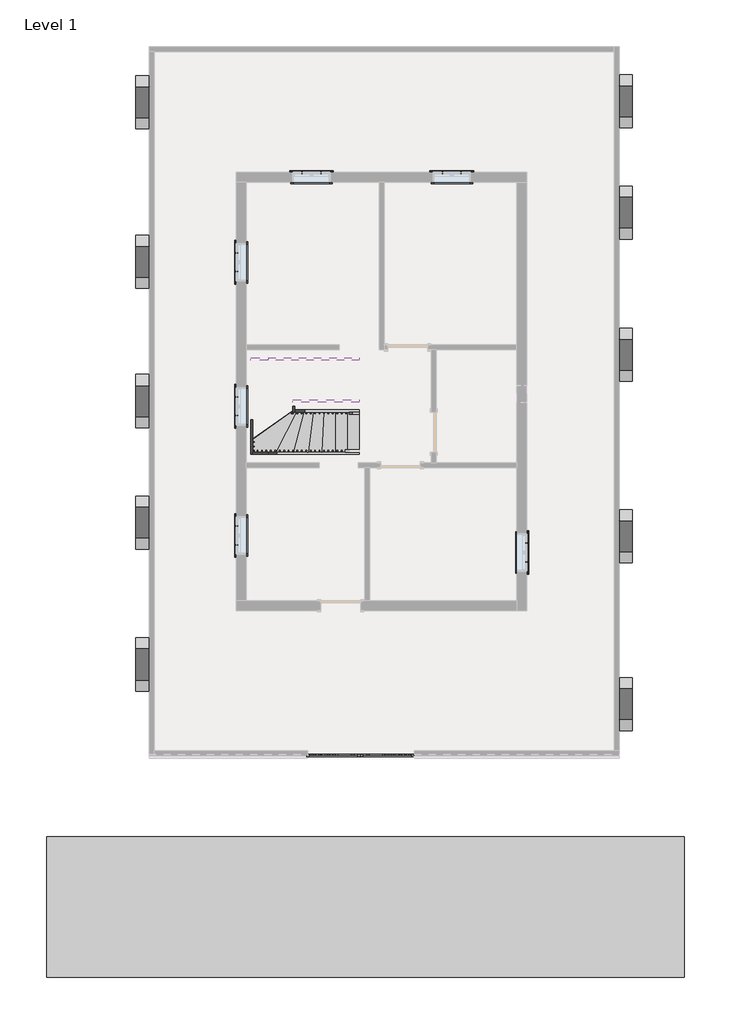
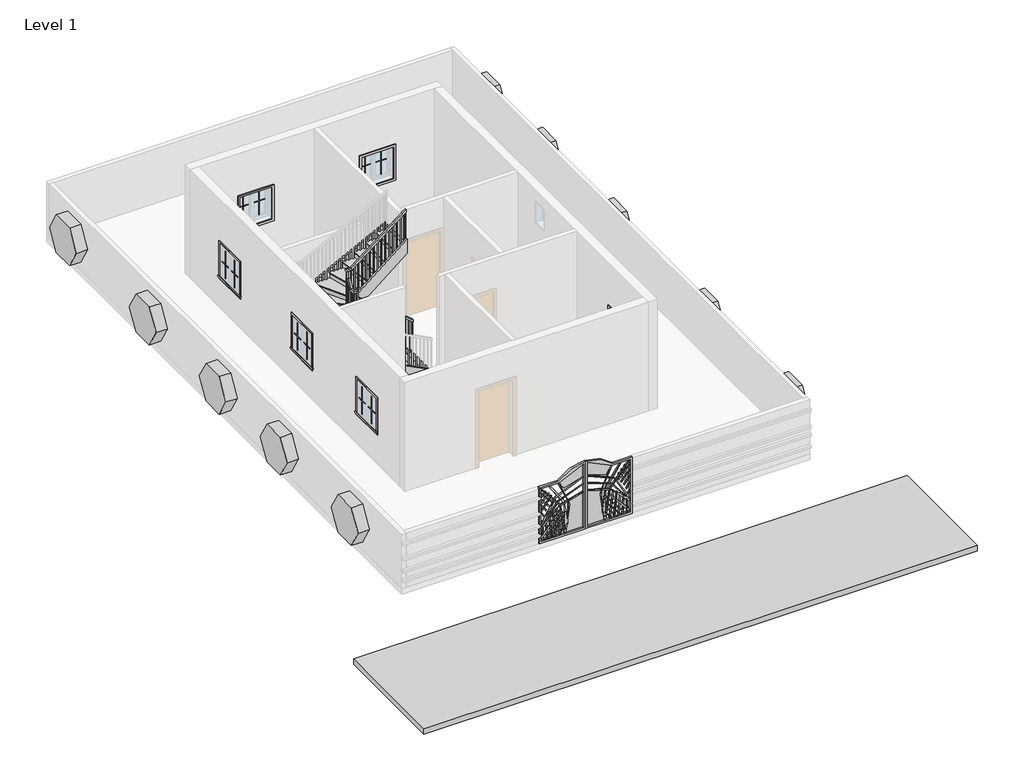
# One storey, part 3 of 3: 28 proxies, 8 members, 1 railing, 1 stair flight.
"""IFC4 building model written with IfcOpenShell, lengths in millimetres."""

from ifc_helpers import new_model, si_unit, frame, origin, place, context, project, spatial, polyline, outline, extrude, faceted_brep, transform, mapped, element, save
from components import generic_models_6bc30956, generic_models_2_generic_models_2_a0eb84b6, generic_models_3_generic_models_3_c1cfd057, generic_models_4_generic_models_4_ada6ec20, muntin_pattern_2x2_muntin_pattern_2x2_b3fe6957, muntin_pattern_2x2_muntin_pattern_2x2_3e0ecaf2, trim_window_exterior_flat_with_sill_41619996, trim_window_interior_flat_picture_frame_51c85655, stair_flight_6f16d7d9

model = new_model("IFC4")

# Units and contexts
model_context = context("Model", 3, world=origin())
ifc_project = project(units=[si_unit("LENGTHUNIT", "METRE", prefix="MILLI")], contexts=[model_context])

# Site, building, storey
site = spatial("IfcSite", under=ifc_project)
building = spatial("IfcBuilding", under=site)
storey = spatial("IfcBuildingStorey", under=building, Name="Level 1", Elevation=0.0)

# Proxies
placement = place(None, origin())
generic_models_shape = generic_models_6bc30956(model_context)
element("IfcBuildingElementProxy", 1, Name="Generic Models", at=placement, inside=storey, context=model_context, shape_type="MappedRepresentation", body=[
    mapped(generic_models_shape, transform((-1768.0949167, -8199.8056704, 0.0), x_axis=(1.0, 0.0, 0.0), y_axis=(0.0, 1.0, 0.0), z_axis=(0.0, 0.0, 1.0))),
])
generic_models_2_generic_models_2_shape = generic_models_2_generic_models_2_a0eb84b6(model_context)
element("IfcBuildingElementProxy", 2, Name="Generic Models 2 : Generic Models 2", ObjectType="Generic Models 2 : Generic Models 2", at=placement, inside=storey, context=model_context, shape_type="MappedRepresentation", body=[
    mapped(generic_models_2_generic_models_2_shape, transform((0.0, 0.0, 0.0), x_axis=(1.0, 0.0, 0.0), y_axis=(0.0, 1.0, 0.0), z_axis=(0.0, 0.0, 1.0))),
])
generic_models_3_generic_models_3_shape = generic_models_3_generic_models_3_c1cfd057(model_context)
element("IfcBuildingElementProxy", 3, Name="Generic Models 3 : Generic Models 3", ObjectType="Generic Models 3 : Generic Models 3", at=placement, inside=storey, context=model_context, shape_type="MappedRepresentation", body=[
    mapped(generic_models_3_generic_models_3_shape, transform((0.0, 0.0, 0.0), x_axis=(1.0, 0.0, 0.0), y_axis=(0.0, 1.0, 0.0), z_axis=(0.0, 0.0, 1.0))),
])
generic_models_4_generic_models_4_shape = generic_models_4_generic_models_4_ada6ec20(model_context)
element("IfcBuildingElementProxy", 4, Name="Generic Models 4 : Generic Models 4", ObjectType="Generic Models 4 : Generic Models 4", at=placement, inside=storey, context=model_context, shape_type="MappedRepresentation", body=[
    mapped(generic_models_4_generic_models_4_shape, transform((0.0, 0.0, 0.0), x_axis=(1.0, 0.0, 0.0), y_axis=(0.0, 1.0, 0.0), z_axis=(0.0, 0.0, 1.0))),
])
muntin_pattern_2x2_muntin_pattern_2x2_shape = muntin_pattern_2x2_muntin_pattern_2x2_b3fe6957(model_context)
element("IfcBuildingElementProxy", 5, Name="Muntin Pattern_2x2 : Muntin Pattern_2x2", ObjectType="Muntin Pattern_2x2 : Muntin Pattern_2x2", at=placement, inside=storey, context=model_context, shape_type="MappedRepresentation", body=[
    mapped(muntin_pattern_2x2_muntin_pattern_2x2_shape, transform((-3096.8324167, 5150.2179147, 984.25), x_axis=(1.0, 0.0, 0.0), y_axis=(0.0, 1.0, 0.0), z_axis=(0.0, 0.0, 1.0))),
])
element("IfcBuildingElementProxy", 6, Name="Muntin Pattern_2x2 : Muntin Pattern_2x2", ObjectType="Muntin Pattern_2x2 : Muntin Pattern_2x2", at=placement, inside=storey, context=model_context, shape_type="MappedRepresentation", body=[
    mapped(muntin_pattern_2x2_muntin_pattern_2x2_shape, transform((122.6175833, 5150.2179147, 984.25), x_axis=(1.0, 0.0, 0.0), y_axis=(0.0, 1.0, 0.0), z_axis=(0.0, 0.0, 1.0))),
])
element("IfcBuildingElementProxy", 7, Name="Muntin Pattern_2x2 : Muntin Pattern_2x2", ObjectType="Muntin Pattern_2x2 : Muntin Pattern_2x2", at=placement, inside=storey, context=model_context, shape_type="MappedRepresentation", body=[
    mapped(muntin_pattern_2x2_muntin_pattern_2x2_shape, transform((2051.4300833, -3350.8445853, 984.25), x_axis=(0.0, -1.0, 0.0), y_axis=(1.0, 0.0, 0.0), z_axis=(0.0, 0.0, 1.0))),
])
element("IfcBuildingElementProxy", 8, Name="Muntin Pattern_2x2 : Muntin Pattern_2x2", ObjectType="Muntin Pattern_2x2 : Muntin Pattern_2x2", at=placement, inside=storey, context=model_context, shape_type="MappedRepresentation", body=[
    mapped(muntin_pattern_2x2_muntin_pattern_2x2_shape, transform((-4597.0199167, -426.6695853, 984.25), x_axis=(0.0, 1.0, 0.0), y_axis=(-1.0, 0.0, 0.0), z_axis=(0.0, 0.0, 1.0))),
])
element("IfcBuildingElementProxy", 9, Name="Muntin Pattern_2x2 : Muntin Pattern_2x2", ObjectType="Muntin Pattern_2x2 : Muntin Pattern_2x2", at=placement, inside=storey, context=model_context, shape_type="MappedRepresentation", body=[
    mapped(muntin_pattern_2x2_muntin_pattern_2x2_shape, transform((-4597.0199167, -3388.9445853, 984.25), x_axis=(0.0, 1.0, 0.0), y_axis=(-1.0, 0.0, 0.0), z_axis=(0.0, 0.0, 1.0))),
])
element("IfcBuildingElementProxy", 10, Name="Muntin Pattern_2x2 : Muntin Pattern_2x2", ObjectType="Muntin Pattern_2x2 : Muntin Pattern_2x2", at=placement, inside=storey, context=model_context, shape_type="MappedRepresentation", body=[
    mapped(muntin_pattern_2x2_muntin_pattern_2x2_shape, transform((-4597.0199167, 2878.5054147, 984.25), x_axis=(0.0, 1.0, 0.0), y_axis=(-1.0, 0.0, 0.0), z_axis=(0.0, 0.0, 1.0))),
])
muntin_pattern_2x2_muntin_pattern_2x2_2_shape = muntin_pattern_2x2_muntin_pattern_2x2_3e0ecaf2(model_context)
element("IfcBuildingElementProxy", 11, Name="Muntin Pattern_2x2 : Muntin Pattern_2x2", ObjectType="Muntin Pattern_2x2 : Muntin Pattern_2x2", at=placement, inside=storey, context=model_context, shape_type="MappedRepresentation", body=[
    mapped(muntin_pattern_2x2_muntin_pattern_2x2_2_shape, transform((-2668.2074167, 5150.2179147, 984.25), x_axis=(-1.0, 0.0, 0.0), y_axis=(0.0, -1.0, 0.0), z_axis=(0.0, 0.0, 1.0))),
])
element("IfcBuildingElementProxy", 12, Name="Muntin Pattern_2x2 : Muntin Pattern_2x2", ObjectType="Muntin Pattern_2x2 : Muntin Pattern_2x2", at=placement, inside=storey, context=model_context, shape_type="MappedRepresentation", body=[
    mapped(muntin_pattern_2x2_muntin_pattern_2x2_2_shape, transform((551.2425833, 5150.2179147, 984.25), x_axis=(-1.0, 0.0, 0.0), y_axis=(0.0, -1.0, 0.0), z_axis=(0.0, 0.0, 1.0))),
])
element("IfcBuildingElementProxy", 13, Name="Muntin Pattern_2x2 : Muntin Pattern_2x2", ObjectType="Muntin Pattern_2x2 : Muntin Pattern_2x2", at=placement, inside=storey, context=model_context, shape_type="MappedRepresentation", body=[
    mapped(muntin_pattern_2x2_muntin_pattern_2x2_2_shape, transform((2051.4300833, -3779.4695853, 984.25), x_axis=(0.0, 1.0, 0.0), y_axis=(-1.0, 0.0, 0.0), z_axis=(0.0, 0.0, 1.0))),
])
element("IfcBuildingElementProxy", 14, Name="Muntin Pattern_2x2 : Muntin Pattern_2x2", ObjectType="Muntin Pattern_2x2 : Muntin Pattern_2x2", at=placement, inside=storey, context=model_context, shape_type="MappedRepresentation", body=[
    mapped(muntin_pattern_2x2_muntin_pattern_2x2_2_shape, transform((-4597.0199167, 1.9554147, 984.25), x_axis=(0.0, -1.0, 0.0), y_axis=(1.0, 0.0, 0.0), z_axis=(0.0, 0.0, 1.0))),
])
element("IfcBuildingElementProxy", 15, Name="Muntin Pattern_2x2 : Muntin Pattern_2x2", ObjectType="Muntin Pattern_2x2 : Muntin Pattern_2x2", at=placement, inside=storey, context=model_context, shape_type="MappedRepresentation", body=[
    mapped(muntin_pattern_2x2_muntin_pattern_2x2_2_shape, transform((-4597.0199167, -2960.3195853, 984.25), x_axis=(0.0, -1.0, 0.0), y_axis=(1.0, 0.0, 0.0), z_axis=(0.0, 0.0, 1.0))),
])
element("IfcBuildingElementProxy", 16, Name="Muntin Pattern_2x2 : Muntin Pattern_2x2", ObjectType="Muntin Pattern_2x2 : Muntin Pattern_2x2", at=placement, inside=storey, context=model_context, shape_type="MappedRepresentation", body=[
    mapped(muntin_pattern_2x2_muntin_pattern_2x2_2_shape, transform((-4597.0199167, 3307.1304147, 984.25), x_axis=(0.0, -1.0, 0.0), y_axis=(1.0, 0.0, 0.0), z_axis=(0.0, 0.0, 1.0))),
])
trim_window_exterior_flat_with_sill_shape = trim_window_exterior_flat_with_sill_41619996(model_context)
element("IfcBuildingElementProxy", 17, Name="Trim-Window-Exterior-Flat : with Sill", ObjectType="Trim-Window-Exterior-Flat : with Sill", at=placement, inside=storey, context=model_context, shape_type="MappedRepresentation", body=[
    mapped(trim_window_exterior_flat_with_sill_shape, transform((-2882.5199167, 5159.7429147, 1828.8), x_axis=(-1.0, 0.0, 0.0), y_axis=(0.0, 0.0, 1.0), z_axis=(0.0, 1.0, 0.0))),
])
element("IfcBuildingElementProxy", 18, Name="Trim-Window-Exterior-Flat : with Sill", ObjectType="Trim-Window-Exterior-Flat : with Sill", at=placement, inside=storey, context=model_context, shape_type="MappedRepresentation", body=[
    mapped(trim_window_exterior_flat_with_sill_shape, transform((336.9300833, 5159.7429147, 1828.8), x_axis=(-1.0, 0.0, 0.0), y_axis=(0.0, 0.0, 1.0), z_axis=(0.0, 1.0, 0.0))),
])
element("IfcBuildingElementProxy", 19, Name="Trim-Window-Exterior-Flat : with Sill", ObjectType="Trim-Window-Exterior-Flat : with Sill", at=placement, inside=storey, context=model_context, shape_type="MappedRepresentation", body=[
    mapped(trim_window_exterior_flat_with_sill_shape, transform((2060.9550833, -3565.1570853, 1828.8), x_axis=(0.0, 1.0, 0.0), y_axis=(0.0, 0.0, 1.0), z_axis=(1.0, 0.0, 0.0))),
])
element("IfcBuildingElementProxy", 20, Name="Trim-Window-Exterior-Flat : with Sill", ObjectType="Trim-Window-Exterior-Flat : with Sill", at=placement, inside=storey, context=model_context, shape_type="MappedRepresentation", body=[
    mapped(trim_window_exterior_flat_with_sill_shape, transform((-4606.5449167, -212.3570853, 1828.8), x_axis=(0.0, -1.0, 0.0), y_axis=(0.0, 0.0, 1.0), z_axis=(-1.0, 0.0, 0.0))),
])
element("IfcBuildingElementProxy", 21, Name="Trim-Window-Exterior-Flat : with Sill", ObjectType="Trim-Window-Exterior-Flat : with Sill", at=placement, inside=storey, context=model_context, shape_type="MappedRepresentation", body=[
    mapped(trim_window_exterior_flat_with_sill_shape, transform((-4606.5449167, -3174.6320853, 1828.8), x_axis=(0.0, -1.0, 0.0), y_axis=(0.0, 0.0, 1.0), z_axis=(-1.0, 0.0, 0.0))),
])
element("IfcBuildingElementProxy", 22, Name="Trim-Window-Exterior-Flat : with Sill", ObjectType="Trim-Window-Exterior-Flat : with Sill", at=placement, inside=storey, context=model_context, shape_type="MappedRepresentation", body=[
    mapped(trim_window_exterior_flat_with_sill_shape, transform((-4606.5449167, 3092.8179147, 1828.8), x_axis=(0.0, -1.0, 0.0), y_axis=(0.0, 0.0, 1.0), z_axis=(-1.0, 0.0, 0.0))),
])
trim_window_interior_flat_picture_frame_shape = trim_window_interior_flat_picture_frame_51c85655(model_context)
element("IfcBuildingElementProxy", 23, Name="Trim-Window-Interior-Flat : Picture Frame", ObjectType="Trim-Window-Interior-Flat : Picture Frame", at=placement, inside=storey, context=model_context, shape_type="MappedRepresentation", body=[
    mapped(trim_window_interior_flat_picture_frame_shape, transform((-2882.5199167, 4931.1429147, 1828.8), x_axis=(1.0, 0.0, 0.0), y_axis=(0.0, 0.0, 1.0), z_axis=(0.0, -1.0, 0.0))),
])
element("IfcBuildingElementProxy", 24, Name="Trim-Window-Interior-Flat : Picture Frame", ObjectType="Trim-Window-Interior-Flat : Picture Frame", at=placement, inside=storey, context=model_context, shape_type="MappedRepresentation", body=[
    mapped(trim_window_interior_flat_picture_frame_shape, transform((336.9300833, 4931.1429147, 1828.8), x_axis=(1.0, 0.0, 0.0), y_axis=(0.0, 0.0, 1.0), z_axis=(0.0, -1.0, 0.0))),
])
element("IfcBuildingElementProxy", 25, Name="Trim-Window-Interior-Flat : Picture Frame", ObjectType="Trim-Window-Interior-Flat : Picture Frame", at=placement, inside=storey, context=model_context, shape_type="MappedRepresentation", body=[
    mapped(trim_window_interior_flat_picture_frame_shape, transform((1832.3550833, -3565.1570853, 1828.8), x_axis=(0.0, -1.0, 0.0), y_axis=(0.0, 0.0, 1.0), z_axis=(-1.0, 0.0, 0.0))),
])
element("IfcBuildingElementProxy", 26, Name="Trim-Window-Interior-Flat : Picture Frame", ObjectType="Trim-Window-Interior-Flat : Picture Frame", at=placement, inside=storey, context=model_context, shape_type="MappedRepresentation", body=[
    mapped(trim_window_interior_flat_picture_frame_shape, transform((-4377.9449167, -212.3570853, 1828.8), x_axis=(0.0, 1.0, 0.0), y_axis=(0.0, 0.0, 1.0), z_axis=(1.0, 0.0, 0.0))),
])
element("IfcBuildingElementProxy", 27, Name="Trim-Window-Interior-Flat : Picture Frame", ObjectType="Trim-Window-Interior-Flat : Picture Frame", at=placement, inside=storey, context=model_context, shape_type="MappedRepresentation", body=[
    mapped(trim_window_interior_flat_picture_frame_shape, transform((-4377.9449167, -3174.6320853, 1828.8), x_axis=(0.0, 1.0, 0.0), y_axis=(0.0, 0.0, 1.0), z_axis=(1.0, 0.0, 0.0))),
])
element("IfcBuildingElementProxy", 28, Name="Trim-Window-Interior-Flat : Picture Frame", ObjectType="Trim-Window-Interior-Flat : Picture Frame", at=placement, inside=storey, context=model_context, shape_type="MappedRepresentation", body=[
    mapped(trim_window_interior_flat_picture_frame_shape, transform((-4377.9449167, 3092.8179147, 1828.8), x_axis=(0.0, 1.0, 0.0), y_axis=(0.0, 0.0, 1.0), z_axis=(1.0, 0.0, 0.0))),
])

# Members
element("IfcMember", 29, ObjectType="Stringer - 2\" Width", at=placement, inside=storey, context=model_context, shape_type="SweptSolid", body=[
    extrude(outline(polyline([(0.0, -1783.4132248), (229.639954, -1783.4132248), (1305.3956453, -3870.8304165), (962.500629, -3870.8304165), (0.0, -2003.1755424), (0.0, -1783.4132248)])), frame((0.0, -1310.9070853, 0.0), z_axis=(0.0, 1.0, 0.0), x_axis=(0.0, 0.0, 1.0)), (0.0, 0.0, 1.0), 50.8),
])
element("IfcMember", 30, ObjectType="Stringer - 2\" Width", at=placement, inside=storey, context=model_context, shape_type="SweptSolid", body=[
    extrude(outline(polyline([(-3870.8304165, -1260.1070853), (-3870.8304165, -1310.9070853), (-4225.5449167, -1310.9070853), (-4225.5449167, -1260.1070853), (-3870.8304165, -1260.1070853)])), frame((0.0, 0.0, 962.500629), z_axis=(0.0, 0.0, 1.0), x_axis=(1.0, 0.0, 0.0)), (0.0, 0.0, 1.0), 342.8950162),
])
element("IfcMember", 31, ObjectType="Stringer - 2\" Width", at=placement, inside=storey, context=model_context, shape_type="SweptSolid", body=[
    extrude(outline(polyline([(-1310.9070853, 1000.5956453), (-1310.9070853, 1289.0952212), (811.1127974, 1969.9972697), (848.0929147, 1969.9972697), (848.0929147, 1638.9682298), (-1141.3846024, 1000.5956453), (-1310.9070853, 1000.5956453)])), frame((-4276.3449167, 0.0, 0.0), z_axis=(1.0, 0.0, 0.0), x_axis=(0.0, 1.0, 0.0)), (0.0, 0.0, 1.0), 50.8),
])
element("IfcMember", 32, ObjectType="Stringer - 2\" Width", at=placement, inside=storey, context=model_context, shape_type="SweptSolid", body=[
    extrude(outline(polyline([(-4276.3449167, 848.0929147), (-4276.3449167, 898.8929147), (-3870.8304165, 898.8929147), (-3870.8304165, 848.0929147), (-4276.3449167, 848.0929147)])), frame((0.0, 0.0, 1649.8904473), z_axis=(0.0, 0.0, 1.0), x_axis=(1.0, 0.0, 0.0)), (0.0, 0.0, 1.0), 320.1068224),
])
element("IfcMember", 33, ObjectType="Stringer - 2\" Width", at=placement, inside=storey, context=model_context, shape_type="SweptSolid", body=[
    extrude(outline(polyline([(1969.9972697, -3870.8304165), (1649.8904473, -3870.8304165), (2725.6461385, -1783.4132248), (3045.7529609, -1783.4132248), (1969.9972697, -3870.8304165)])), frame((0.0, 848.0929147, 0.0), z_axis=(0.0, 1.0, 0.0), x_axis=(0.0, 0.0, 1.0)), (0.0, 0.0, 1.0), 50.8),
])
element("IfcMember", 34, ObjectType="Stringer - 2\" Width", at=placement, inside=storey, context=model_context, shape_type="SweptSolid", body=[
    extrude(outline(polyline([(0.0, -1783.4132248), (176.1764461, -1783.4132248), (1380.418648, -3260.3449167), (987.1410923, -3260.3449167), (0.0, -2049.6748694), (0.0, -1783.4132248)])), frame((0.0, -345.7070853, 0.0), z_axis=(0.0, 1.0, 0.0), x_axis=(0.0, 0.0, 1.0)), (0.0, 0.0, 1.0), 50.8),
])
element("IfcMember", 35, ObjectType="Stringer - 2\" Width", at=placement, inside=storey, context=model_context, shape_type="SweptSolid", body=[
    extrude(outline(polyline([(-345.7070853, 1028.5617647), (-345.7070853, 1573.2682978), (-139.0699679, 1926.1409689), (-117.1070853, 1926.1409689), (-117.1070853, 1360.465107), (-311.464868, 1028.5617647), (-345.7070853, 1028.5617647)])), frame((-3311.1449167, 0.0, 0.0), z_axis=(1.0, 0.0, 0.0), x_axis=(0.0, 1.0, 0.0)), (0.0, 0.0, 1.0), 50.8),
])
element("IfcMember", 36, ObjectType="Stringer - 2\" Width", at=placement, inside=storey, context=model_context, shape_type="SweptSolid", body=[
    extrude(outline(polyline([(1926.1409689, -3311.1449167), (1532.8634131, -3311.1449167), (2778.5262875, -1783.4132248), (3171.8038432, -1783.4132248), (1926.1409689, -3311.1449167)])), frame((0.0, -117.1070853, 0.0), z_axis=(0.0, 1.0, 0.0), x_axis=(0.0, 0.0, 1.0)), (0.0, 0.0, 1.0), 50.8),
])

# Railing
element("IfcRailing", 37, ObjectType="Handrail - Rectangular", at=placement, inside=storey, context=model_context, shape_type="SolidModel", body=[
    faceted_brep([(-1783.4132248, -396.5070853, 1083.7333333), (-1783.4132248, -396.5070853, 1019.4000346), (-1783.4132248, -345.7070853, 1019.4000346), (-1783.4132248, -345.7070853, 1083.7333333), (-3234.9449167, -396.5070853, 2211.6191036), (-3285.7449167, -396.5070853, 2186.7590024), (-3285.7449167, -345.7070853, 2186.7590024), (-3234.9449167, -345.7070853, 2211.6191036), (-3234.9449167, -396.5070853, 2414.6281882), (-3285.7449167, -396.5070853, 2363.8281882), (-3285.7449167, -345.7070853, 2363.8281882), (-3234.9449167, -345.7070853, 2414.6281882), (-3361.9449167, -396.5070853, 2414.6281882), (-3361.9449167, -396.5070853, 2363.8281882), (-3311.1449167, -345.7070853, 2363.8281882), (-3311.1449167, -345.7070853, 2414.6281882), (-3361.9449167, -269.5070853, 2414.6281882), (-3361.9449167, -240.3857515, 2363.8281882), (-3311.1449167, -240.3857515, 2363.8281882), (-3311.1449167, -269.5070853, 2414.6281882), (-3361.9449167, -142.5070853, 2631.5051451), (-3361.9449167, -91.7070853, 2617.7256424), (-3311.1449167, -91.7070853, 2617.7256424), (-3311.1449167, -142.5070853, 2631.5051451), (-3361.9449167, -142.5070853, 2834.5142297), (-3361.9449167, -91.7070853, 2783.7142297), (-3311.1449167, -91.7070853, 2783.7142297), (-3311.1449167, -142.5070853, 2834.5142297), (-3361.9449167, -15.5070853, 2834.5142297), (-3361.9449167, -15.5070853, 2783.7142297), (-3311.1449167, -66.3070853, 2783.7142297), (-3311.1449167, -66.3070853, 2834.5142297), (-3234.9449167, -15.5070853, 2834.5142297), (-3217.5282487, -15.5070853, 2783.7142297), (-3217.5282487, -66.3070853, 2783.7142297), (-3234.9449167, -66.3070853, 2834.5142297), (-1783.4132248, -15.5070853, 3962.4), (-1783.4132248, -66.3070853, 3962.4), (-1783.4132248, -66.3070853, 3898.0667013), (-1783.4132248, -15.5070853, 3898.0667013)], [[[0, 1, 2, 3]], [[1, 0, 4, 5]], [[2, 1, 5, 6]], [[3, 2, 6, 7]], [[0, 3, 7, 4]], [[5, 4, 8, 9]], [[6, 5, 9, 10]], [[7, 6, 10, 11]], [[4, 7, 11, 8]], [[9, 8, 12, 13]], [[10, 9, 13, 14]], [[11, 10, 14, 15]], [[8, 11, 15, 12]], [[13, 12, 16, 17]], [[14, 13, 17, 18]], [[15, 14, 18, 19]], [[12, 15, 19, 16]], [[17, 16, 20, 21]], [[18, 17, 21, 22]], [[19, 18, 22, 23]], [[16, 19, 23, 20]], [[21, 20, 24, 25]], [[22, 21, 25, 26]], [[23, 22, 26, 27]], [[20, 23, 27, 24]], [[25, 24, 28, 29]], [[26, 25, 29, 30]], [[27, 26, 30, 31]], [[24, 27, 31, 28]], [[29, 28, 32, 33]], [[30, 29, 33, 34]], [[31, 30, 34, 35]], [[28, 31, 35, 32]], [[36, 37, 38, 39]], [[33, 32, 36, 39]], [[34, 33, 39, 38]], [[35, 34, 38, 37]], [[32, 35, 37, 36]]]),
    extrude(outline(polyline([(3882.8316852, -1803.0199167), (3868.0292361, -1822.0699167), (2878.6666667, -1822.0699167), (2878.6666667, -1803.0199167), (3882.8316852, -1803.0199167)])), frame((0.0, -50.4320853, 0.0), z_axis=(0.0, 1.0, 0.0), x_axis=(0.0, 0.0, 1.0)), (0.0, 0.0, 1.0), 19.05),
    extrude(outline(polyline([(3803.8852902, -1904.6199167), (3789.0828411, -1923.6699167), (2878.6666667, -1923.6699167), (2878.6666667, -1904.6199167), (3803.8852902, -1904.6199167)])), frame((0.0, -50.4320853, 0.0), z_axis=(0.0, 1.0, 0.0), x_axis=(0.0, 0.0, 1.0)), (0.0, 0.0, 1.0), 19.05),
    extrude(outline(polyline([(3724.9388952, -2006.2199167), (3710.1364462, -2025.2699167), (2878.6666667, -2025.2699167), (2878.6666667, -2006.2199167), (3724.9388952, -2006.2199167)])), frame((0.0, -50.4320853, 0.0), z_axis=(0.0, 1.0, 0.0), x_axis=(0.0, 0.0, 1.0)), (0.0, 0.0, 1.0), 19.05),
    extrude(outline(polyline([(3645.9925003, -2107.8199167), (3631.1900512, -2126.8699167), (2709.3333333, -2126.8699167), (2709.3333333, -2107.8199167), (3645.9925003, -2107.8199167)])), frame((0.0, -50.4320853, 0.0), z_axis=(0.0, 1.0, 0.0), x_axis=(0.0, 0.0, 1.0)), (0.0, 0.0, 1.0), 19.05),
    extrude(outline(polyline([(3567.0461053, -2209.4199167), (3552.2436562, -2228.4699167), (2709.3333333, -2228.4699167), (2709.3333333, -2209.4199167), (3567.0461053, -2209.4199167)])), frame((0.0, -50.4320853, 0.0), z_axis=(0.0, 1.0, 0.0), x_axis=(0.0, 0.0, 1.0)), (0.0, 0.0, 1.0), 19.05),
    extrude(outline(polyline([(3488.0997103, -2311.0199167), (3473.2972613, -2330.0699167), (2709.3333333, -2330.0699167), (2709.3333333, -2311.0199167), (3488.0997103, -2311.0199167)])), frame((0.0, -50.4320853, 0.0), z_axis=(0.0, 1.0, 0.0), x_axis=(0.0, 0.0, 1.0)), (0.0, 0.0, 1.0), 19.05),
    extrude(outline(polyline([(3409.1533154, -2412.6199167), (3394.3508663, -2431.6699167), (2540.0, -2431.6699167), (2540.0, -2412.6199167), (3409.1533154, -2412.6199167)])), frame((0.0, -50.4320853, 0.0), z_axis=(0.0, 1.0, 0.0), x_axis=(0.0, 0.0, 1.0)), (0.0, 0.0, 1.0), 19.05),
    extrude(outline(polyline([(3330.2069204, -2514.2199167), (3315.4044713, -2533.2699167), (2540.0, -2533.2699167), (2540.0, -2514.2199167), (3330.2069204, -2514.2199167)])), frame((0.0, -50.4320853, 0.0), z_axis=(0.0, 1.0, 0.0), x_axis=(0.0, 0.0, 1.0)), (0.0, 0.0, 1.0), 19.05),
    extrude(outline(polyline([(3251.2605254, -2615.8199167), (3236.4580764, -2634.8699167), (2370.6666667, -2634.8699167), (2370.6666667, -2615.8199167), (3251.2605254, -2615.8199167)])), frame((0.0, -50.4320853, 0.0), z_axis=(0.0, 1.0, 0.0), x_axis=(0.0, 0.0, 1.0)), (0.0, 0.0, 1.0), 19.05),
    extrude(outline(polyline([(3172.3141304, -2717.4199167), (3157.5116814, -2736.4699167), (2370.6666667, -2736.4699167), (2370.6666667, -2717.4199167), (3172.3141304, -2717.4199167)])), frame((0.0, -50.4320853, 0.0), z_axis=(0.0, 1.0, 0.0), x_axis=(0.0, 0.0, 1.0)), (0.0, 0.0, 1.0), 19.05),
    extrude(outline(polyline([(3093.3677355, -2819.0199167), (3078.5652864, -2838.0699167), (2370.6666667, -2838.0699167), (2370.6666667, -2819.0199167), (3093.3677355, -2819.0199167)])), frame((0.0, -50.4320853, 0.0), z_axis=(0.0, 1.0, 0.0), x_axis=(0.0, 0.0, 1.0)), (0.0, 0.0, 1.0), 19.05),
    extrude(outline(polyline([(3014.4213405, -2920.6199167), (2999.6188914, -2939.6699167), (2201.3333333, -2939.6699167), (2201.3333333, -2920.6199167), (3014.4213405, -2920.6199167)])), frame((0.0, -50.4320853, 0.0), z_axis=(0.0, 1.0, 0.0), x_axis=(0.0, 0.0, 1.0)), (0.0, 0.0, 1.0), 19.05),
    extrude(outline(polyline([(2935.4749455, -3022.2199167), (2920.6724965, -3041.2699167), (2201.3333333, -3041.2699167), (2201.3333333, -3022.2199167), (2935.4749455, -3022.2199167)])), frame((0.0, -50.4320853, 0.0), z_axis=(0.0, 1.0, 0.0), x_axis=(0.0, 0.0, 1.0)), (0.0, 0.0, 1.0), 19.05),
    extrude(outline(polyline([(2856.5285506, -3123.8199167), (2841.7261015, -3142.8699167), (2032.0, -3142.8699167), (2032.0, -3123.8199167), (2856.5285506, -3123.8199167)])), frame((0.0, -50.4320853, 0.0), z_axis=(0.0, 1.0, 0.0), x_axis=(0.0, 0.0, 1.0)), (0.0, 0.0, 1.0), 19.05),
    extrude(outline(polyline([(2777.5821556, -3225.4199167), (2762.7797065, -3244.4699167), (2032.0, -3244.4699167), (2032.0, -3225.4199167), (2777.5821556, -3225.4199167)])), frame((0.0, -50.4320853, 0.0), z_axis=(0.0, 1.0, 0.0), x_axis=(0.0, 0.0, 1.0)), (0.0, 0.0, 1.0), 19.05),
    extrude(outline(polyline([(-3327.0199167, -75.8320853), (-3346.0699167, -75.8320853), (-3346.0699167, -56.7820853), (-3327.0199167, -56.7820853), (-3327.0199167, -75.8320853)])), frame((0.0, 0.0, 1693.3333333), z_axis=(0.0, 0.0, 1.0), x_axis=(1.0, 0.0, 0.0)), (0.0, 0.0, 1.0), 1090.3808964),
    extrude(outline(polyline([(-177.4320853, 2471.3336964), (-158.3820853, 2503.86524), (-158.3820853, 1524.0), (-177.4320853, 1524.0), (-177.4320853, 2471.3336964)])), frame((-3346.0699167, 0.0, 0.0), z_axis=(1.0, 0.0, 0.0), x_axis=(0.0, 1.0, 0.0)), (0.0, 0.0, 1.0), 19.05),
    extrude(outline(polyline([(-279.0320853, 2297.8321309), (-259.9820853, 2330.3636744), (-259.9820853, 1354.6666667), (-279.0320853, 1354.6666667), (-279.0320853, 2297.8321309)])), frame((-3346.0699167, 0.0, 0.0), z_axis=(1.0, 0.0, 0.0), x_axis=(0.0, 1.0, 0.0)), (0.0, 0.0, 1.0), 19.05),
    extrude(outline(polyline([(-3297.8882248, -361.5820853), (-3297.8882248, -380.6320853), (-3316.9382248, -380.6320853), (-3316.9382248, -361.5820853), (-3297.8882248, -361.5820853)])), frame((0.0, 0.0, 1185.3333333), z_axis=(0.0, 0.0, 1.0), x_axis=(1.0, 0.0, 0.0)), (0.0, 0.0, 1.0), 1178.4948549),
    extrude(outline(polyline([(2117.2483397, -3196.2882248), (2132.0507888, -3215.3382248), (1016.0, -3215.3382248), (1016.0, -3196.2882248), (2117.2483397, -3196.2882248)])), frame((0.0, -380.6320853, 0.0), z_axis=(0.0, 1.0, 0.0), x_axis=(0.0, 0.0, 1.0)), (0.0, 0.0, 1.0), 19.05),
    extrude(outline(polyline([(2038.3019447, -3094.6882248), (2053.1043938, -3113.7382248), (1016.0, -3113.7382248), (1016.0, -3094.6882248), (2038.3019447, -3094.6882248)])), frame((0.0, -380.6320853, 0.0), z_axis=(0.0, 1.0, 0.0), x_axis=(0.0, 0.0, 1.0)), (0.0, 0.0, 1.0), 19.05),
    extrude(outline(polyline([(1959.3555498, -2993.0882248), (1974.1579988, -3012.1382248), (846.6666667, -3012.1382248), (846.6666667, -2993.0882248), (1959.3555498, -2993.0882248)])), frame((0.0, -380.6320853, 0.0), z_axis=(0.0, 1.0, 0.0), x_axis=(0.0, 0.0, 1.0)), (0.0, 0.0, 1.0), 19.05),
    extrude(outline(polyline([(1880.4091548, -2891.4882248), (1895.2116039, -2910.5382248), (846.6666667, -2910.5382248), (846.6666667, -2891.4882248), (1880.4091548, -2891.4882248)])), frame((0.0, -380.6320853, 0.0), z_axis=(0.0, 1.0, 0.0), x_axis=(0.0, 0.0, 1.0)), (0.0, 0.0, 1.0), 19.05),
    extrude(outline(polyline([(1801.4627598, -2789.8882248), (1816.2652089, -2808.9382248), (677.3333333, -2808.9382248), (677.3333333, -2789.8882248), (1801.4627598, -2789.8882248)])), frame((0.0, -380.6320853, 0.0), z_axis=(0.0, 1.0, 0.0), x_axis=(0.0, 0.0, 1.0)), (0.0, 0.0, 1.0), 19.05),
    extrude(outline(polyline([(1722.5163649, -2688.2882248), (1737.3188139, -2707.3382248), (677.3333333, -2707.3382248), (677.3333333, -2688.2882248), (1722.5163649, -2688.2882248)])), frame((0.0, -380.6320853, 0.0), z_axis=(0.0, 1.0, 0.0), x_axis=(0.0, 0.0, 1.0)), (0.0, 0.0, 1.0), 19.05),
    extrude(outline(polyline([(1643.5699699, -2586.6882248), (1658.3724189, -2605.7382248), (508.0, -2605.7382248), (508.0, -2586.6882248), (1643.5699699, -2586.6882248)])), frame((0.0, -380.6320853, 0.0), z_axis=(0.0, 1.0, 0.0), x_axis=(0.0, 0.0, 1.0)), (0.0, 0.0, 1.0), 19.05),
    extrude(outline(polyline([(1564.6235749, -2485.0882248), (1579.426024, -2504.1382248), (508.0, -2504.1382248), (508.0, -2485.0882248), (1564.6235749, -2485.0882248)])), frame((0.0, -380.6320853, 0.0), z_axis=(0.0, 1.0, 0.0), x_axis=(0.0, 0.0, 1.0)), (0.0, 0.0, 1.0), 19.05),
    extrude(outline(polyline([(1485.6771799, -2383.4882248), (1500.479629, -2402.5382248), (508.0, -2402.5382248), (508.0, -2383.4882248), (1485.6771799, -2383.4882248)])), frame((0.0, -380.6320853, 0.0), z_axis=(0.0, 1.0, 0.0), x_axis=(0.0, 0.0, 1.0)), (0.0, 0.0, 1.0), 19.05),
    extrude(outline(polyline([(1406.730785, -2281.8882248), (1421.533234, -2300.9382248), (338.6666667, -2300.9382248), (338.6666667, -2281.8882248), (1406.730785, -2281.8882248)])), frame((0.0, -380.6320853, 0.0), z_axis=(0.0, 1.0, 0.0), x_axis=(0.0, 0.0, 1.0)), (0.0, 0.0, 1.0), 19.05),
    extrude(outline(polyline([(1327.78439, -2180.2882248), (1342.5868391, -2199.3382248), (338.6666667, -2199.3382248), (338.6666667, -2180.2882248), (1327.78439, -2180.2882248)])), frame((0.0, -380.6320853, 0.0), z_axis=(0.0, 1.0, 0.0), x_axis=(0.0, 0.0, 1.0)), (0.0, 0.0, 1.0), 19.05),
    extrude(outline(polyline([(1248.837995, -2078.6882248), (1263.6404441, -2097.7382248), (338.6666667, -2097.7382248), (338.6666667, -2078.6882248), (1248.837995, -2078.6882248)])), frame((0.0, -380.6320853, 0.0), z_axis=(0.0, 1.0, 0.0), x_axis=(0.0, 0.0, 1.0)), (0.0, 0.0, 1.0), 19.05),
    extrude(outline(polyline([(1169.8916001, -1977.0882248), (1184.6940491, -1996.1382248), (169.3333333, -1996.1382248), (169.3333333, -1977.0882248), (1169.8916001, -1977.0882248)])), frame((0.0, -380.6320853, 0.0), z_axis=(0.0, 1.0, 0.0), x_axis=(0.0, 0.0, 1.0)), (0.0, 0.0, 1.0), 19.05),
    extrude(outline(polyline([(1090.9452051, -1875.4882248), (1105.7476541, -1894.5382248), (169.3333333, -1894.5382248), (169.3333333, -1875.4882248), (1090.9452051, -1875.4882248)])), frame((0.0, -380.6320853, 0.0), z_axis=(0.0, 1.0, 0.0), x_axis=(0.0, 0.0, 1.0)), (0.0, 0.0, 1.0), 19.05),
    extrude(outline(polyline([(-3327.0199167, -50.4320853), (-3346.0699167, -50.4320853), (-3346.0699167, -31.3820853), (-3327.0199167, -31.3820853), (-3327.0199167, -50.4320853)])), frame((0.0, 0.0, 1862.6666667), z_axis=(0.0, 0.0, 1.0), x_axis=(1.0, 0.0, 0.0)), (0.0, 0.0, 1.0), 921.0475631),
    extrude(outline(polyline([(-3327.0199167, -361.5820853), (-3327.0199167, -380.6320853), (-3346.0699167, -380.6320853), (-3346.0699167, -361.5820853), (-3327.0199167, -361.5820853)])), frame((0.0, 0.0, 1185.3333333), z_axis=(0.0, 0.0, 1.0), x_axis=(1.0, 0.0, 0.0)), (0.0, 0.0, 1.0), 1178.4948549),
    extrude(outline(polyline([(3898.0667013, -1783.4132248), (3883.2642523, -1802.4632248), (2878.6666667, -1802.4632248), (2878.6666667, -1783.4132248), (3898.0667013, -1783.4132248)])), frame((0.0, -50.4320853, 0.0), z_axis=(0.0, 1.0, 0.0), x_axis=(0.0, 0.0, 1.0)), (0.0, 0.0, 1.0), 19.05),
    extrude(outline(polyline([(1019.4000346, -1783.4132248), (1034.2024837, -1802.4632248), (169.3333333, -1802.4632248), (169.3333333, -1783.4132248), (1019.4000346, -1783.4132248)])), frame((0.0, -380.6320853, 0.0), z_axis=(0.0, 1.0, 0.0), x_axis=(0.0, 0.0, 1.0)), (0.0, 0.0, 1.0), 19.05),
])

# Stair flight
stair_flight_shape = stair_flight_6f16d7d9(model_context)
element("IfcStairFlight", 38, ObjectType="2\" Tread 1\" Nosing 1/4\" Riser", at=placement, inside=storey, context=model_context, shape_type="MappedRepresentation", body=[
    mapped(stair_flight_shape, transform((0.0, 0.0, 0.0), x_axis=(1.0, 0.0, 0.0), y_axis=(0.0, 1.0, 0.0), z_axis=(0.0, 0.0, 1.0))),
])

save(model, "model.ifc")

# Revit data of these elements
# Type
#   m.s. sheet = none
#   2" x2" pipe = none
#   1"x1"pipe = none
#   Default Elevation = 0
# Type "Muntin Pattern_2x2 : Muntin Pattern_2x2"
#   Width [instance default] = 4' - 0"
#   Thickness = 0' - 0 1/2"
#   Height [instance default] = 4' - 0"
#   Distance = 0' - 0 3/4"
#   Interior Material [instance default] = none
#   Exterior Material [instance default] = none
#   Default Elevation = 0
# Type "Trim-Window-Exterior-Flat : with Sill"
#   Trim Width = 0' - 2 1/4"
#   Trim Thickness_Picture Frame = 0' - 1 1/4"
#   Trim Thickness_with Sill = 0' - 0 3/4"
#   Sill Thickness = 0' - 1 1/4"
#   Opening Width [instance default] = 2' - 0"
#   Opening Height [instance default] = 3' - 0"
#   Default Elevation = 4' - 0"
#   Sill = yes
#   Picture Frame = no
#   Trim Material [instance default] = none
# Type "Trim-Window-Interior-Flat : Picture Frame"
#   Trim Thickness_Picture Frame = 0' - 1 1/4"
#   Trim Width = 0' - 2 1/4"
#   Trim Thickness_with Sill = 0' - 0 3/4"
#   Sill Thickness = 0' - 1 1/4"
#   Opening Width [instance default] = 2' - 0"
#   Opening Height [instance default] = 3' - 0"
#   Default Elevation = 4' - 0"
#   Sill = no
#   Picture Frame = yes
#   Trim Material [instance default] = none
# Type "Handrail - Rectangular"
#   Assembly Code = "C2010400"
#   built-in parameter 1008612 = 0.0416667 (stored number, unit not read)
#   built-in parameter 1008611 = 0.0416667 (stored number, unit not read)
#   built-in parameter 1008609 = 0.333333 (stored number, unit not read)
#   built-in parameter 1008604 = 0.166667 (stored number, unit not read)
#   built-in parameter 1008603 = 0.166667 (stored number, unit not read)
#   Railing Height = 3' - 0"
#   built-in parameter 1008630 = 2
#   built-in parameter 1008610 = 2
#   built-in parameter 1008618 = Baluster - Square : 3/4"
# Element 1 (IfcBuildingElementProxy)
#   Phase Created = New Construction
#   Materials on its faces: "r1"
# Element 2 (IfcBuildingElementProxy, "Generic Models 2 : Generic Models 2")
#   Phase Created = New Construction
#   Materials on its faces: "Clad - White", "Concrete Masonry Units"
# Element 3 (IfcBuildingElementProxy, "Generic Models 3 : Generic Models 3")
#   Phase Created = New Construction
#   Materials on its faces: "Clad - White", "Concrete Masonry Units"
# Element 4 (IfcBuildingElementProxy, "Generic Models 4 : Generic Models 4")
#   Phase Created = New Construction
# Elements 5, 6, 7, 8, 9, 10, 11, 12, 13, 14, 15, 16 (IfcBuildingElementProxy, "Muntin Pattern_2x2 : Muntin Pattern_2x2")
#   Width = 0' - 11 5/8"
#   Height = 2' - 6 1/2"
#   Interior Material = Wood - Stained
#   Exterior Material = Clad - White
#   Phase Created = New Construction
#   Materials on its faces: "Clad - White", "Wood - Stained"
# Elements 17, 18, 19, 20, 21, 22 (IfcBuildingElementProxy, "Trim-Window-Exterior-Flat : with Sill")
#   Opening Width = 2' - 10"
#   Opening Height = 3' - 0"
#   Trim Material = Clad - White
#   Phase Created = New Construction
#   Materials on its faces: "Clad - White"
# Elements 23, 24, 25, 26, 27, 28 (IfcBuildingElementProxy, "Trim-Window-Interior-Flat : Picture Frame")
#   Opening Width = 2' - 10"
#   Opening Height = 3' - 0"
#   Trim Material = Wood - Stained
#   Phase Created = New Construction
#   Materials on its faces: "Wood - Stained"
# Elements 29, 30, 31, 32, 33, 34, 35, 36 (IfcMember, "Stringer - 2\" Width")
#   Phase Created = New Construction
# Element 37 (IfcRailing, "Handrail - Rectangular")
#   Phase Created = New Construction
# Element 38 (IfcStairFlight, "2\" Tread 1\" Nosing 1/4\" Riser")
#   Phase Created = New Construction
# Materials
#   "r1": class "Generic", colour RGB 120 120 120, transparency 0, Cost = 0
#   "Clad - White": class "Wood", colour RGB 242 242 238, transparency 0, Cost = 0
#   "Concrete Masonry Units": class "Masonry", colour RGB 227 227 227, transparency 0, Description = "Concrete masonry units", Cost = 0
#   "Wood - Stained": class "Wood", colour RGB 224 178 126, transparency 0, Cost = 0
